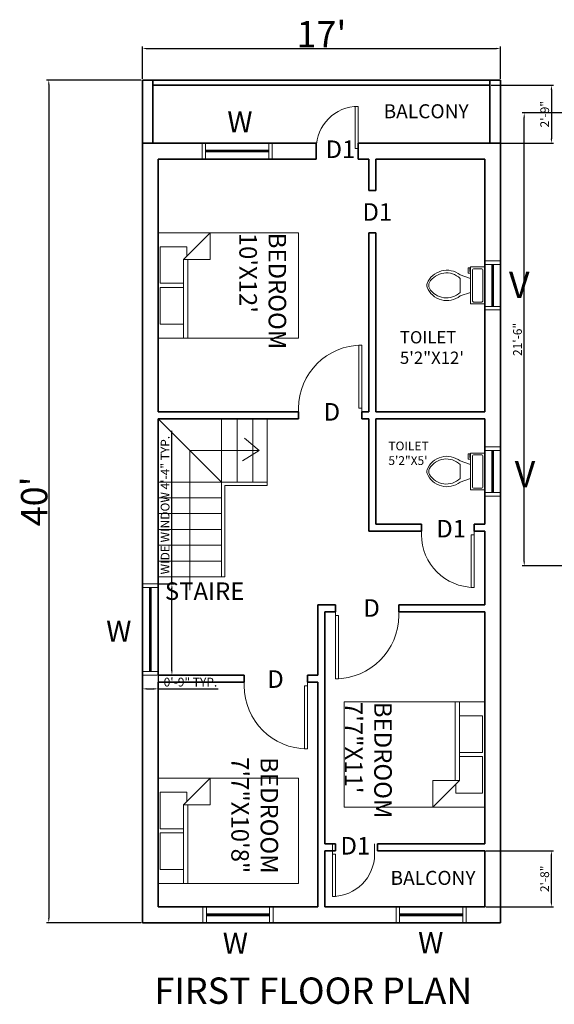
# Model space of a CAD drawing. Units: inches. Extents: x 1662 to 23131, y 1265 to 19127.
# Tile 16 of 26: x 19746 to 20050, y 8212 to 8773. Entities that reach past the tile are written whole.
import ezdxf

# ---------------------------------------------------------------- set-up
doc = ezdxf.new("R2010")
doc.units = ezdxf.units.IN
for name, color, linetype, lineweight in [('A-ANNO-DIMS', 4, 'Continuous', 18), ('A-ANNO-IDEN', 7, 'Continuous', 18), ('A-ANNO-TITL', 7, 'Continuous', 35), ('A-AREA-IDEN', 7, 'Continuous', 18), ('A-DOOR', 3, 'Continuous', 18), ('A-FLOR-FIXT', 9, 'Continuous', 18), ('A-FLOR-STRS', 7, 'Continuous', 18), ('A-FURN', 8, 'Continuous', 18), ('A-GLAZ', 4, 'Continuous', 18), ('A-WALL', 7, 'Continuous', 35)]:
    doc.layers.add(name, color=color, linetype=linetype, lineweight=lineweight)
doc.styles.get("Standard").update_dxf_attribs({"font": 'arial.ttf'})
doc.dimstyles.new('ISO-25', dxfattribs={"dimtxt": 5, "dimasz": 2.5, "dimexe": 1.25, "dimexo": 0.625, "dimtad": 1, "dimlunit": 3, "dimtxsty": 'Standard', "dimcen": 2.5, "dimadec": 0, "dimazin": 0, "dimtfac": 1, "dimtmove": 0, "dimatfit": 3, "dimfxl": 1, "dimarcsym": 0})

# ---------------------------------------------------------------- blocks, each defined once
blk = doc.blocks.new('Bed - Queen')
for p, q in [((0, -80.00003), (0, 0)), ((0, 0), (59.99999, 0)), ((59.99999, 0), (59.99999, -80.00003)), ((7.99999, -1.2), (28.79998, -1.2)), ((7.99999, -14.4), (7.99999, -1.2)), ((28.79998, -1.2), (28.79998, -14.4)), ((31.19999, -1.2), (51.99999, -1.2)), ((31.19999, -14.4), (31.19999, -1.2)), ((51.99999, -1.2), (51.99999, -16.4)), ((0, -14.4), (44.8, -14.4)), ((44.8, -16.8), (0, -16.8)), ((59.99999, -29.6), (44.8, -14.4)), ((44.8, -14.4), (44.8, -29.6)), ((51.99999, -16.4), (46.79936, -16.4)), ((44.8, -29.6), (59.99999, -29.6)), ((59.99999, -80.00003), (0, -80.00003))]:
    blk.add_line(p, q)
blk = doc.blocks.new('Toilet - top')
for p, q in [((9.5, -6), (9.5, -2)), ((-10, -8.5), (-8, -8.5)), ((-10, -9.5), (-10, -8.5)), ((-7, -9.5), (-10, -9.5)), ((-8, -8.5), (-8, -8)), ((-7, -8), (-7, -9.5)), ((-4, -8), (-6, -14)), ((4, -8), (6, -14)), ((4, -14), (-4, -14))]:
    blk.add_line(p, q)
blk.add_lwpolyline([(10.5, -8), (10.5, 0), (-10.5, 0), (-10.5, -8)], close=True)
for points in [[(-9.5, -2), (-9.5, -6)], [(8.5, -1), (-8.5, -1)], [(-8.5, -7), (8.5, -7)]]:
    blk.add_lwpolyline(points)
for centre, radius, start, end in [((-8.62, -1.88), 0.884, 81.8699, 188.1301), ((8.62, -1.88), 0.884, 351.8699, 98.1301), ((-8.62, -6.12), 0.884, 171.8699, 278.1301), ((8.62, -6.12), 0.884, 261.8699, 8.1301), ((3.52, -21.58), 12.17, 141.4691, 247.9714), ((4.2, -21.82), 11.33, 136.3677, 238.9468), ((-3.52, -21.58), 12.17, 292.0284, 38.5307), ((-4.2, -21.82), 11.33, 301.053, 43.6321), ((0, -27.88), 4, 245.7318, 294.2682), ((0, -29), 4, 254.8605, 285.1395)]:
    blk.add_arc(centre, radius, start, end)
blk = doc.blocks.new('*U87')
for p, q in [((-36, 0), (-36, 6)), ((0, 0), (0, 6))]:
    blk.add_line(p, q)
blk.add_lwpolyline([(0, 0), (0, -36), (-1.75, -36), (-1.75, 0)], close=True)
blk.add_arc((0, 0), 36, 180, 270)
blk = doc.blocks.new('*U88')
for p, q in [((0, 0), (0, 6)), ((36, 0), (36, 6))]:
    blk.add_line(p, q)
blk.add_lwpolyline([(0, 0), (0, -36), (1.75, -36), (1.75, 0)], close=True)
blk.add_arc((0, 0), 36, 270, 0)
blk = doc.blocks.new('*U89')
for p, q in [((-36, 0), (-36, -6)), ((0, 0), (0, -6))]:
    blk.add_line(p, q)
blk.add_lwpolyline([(0, 0), (0, 36), (-1.75, 36), (-1.75, 0)], close=True)
blk.add_arc((0, 0), 36, 90, 180)
blk = doc.blocks.new('*U90')
for p, q in [((0, 0), (0, 6)), ((24, 0), (24, 6))]:
    blk.add_line(p, q)
blk.add_lwpolyline([(0, 0), (0, -24), (1.75, -24), (1.75, 0)], close=True)
blk.add_arc((0, 0), 24, 270, 0)
blk = doc.blocks.new('*U91')
for p, q in [((-24, 0), (-24, -6)), ((0, 0), (0, -6))]:
    blk.add_line(p, q)
blk.add_lwpolyline([(0, 0), (0, 24), (-1.75, 24), (-1.75, 0)], close=True)
blk.add_arc((0, 0), 24, 90, 180)
blk = doc.blocks.new('*U92')
for p, q in [((-30, 0), (-30, 6)), ((0, 0), (0, 6))]:
    blk.add_line(p, q)
blk.add_lwpolyline([(0, 0), (0, -30), (-1.75, -30), (-1.75, 0)], close=True)
blk.add_arc((0, 0), 30, 180, 270)
blk = doc.blocks.new('*D96')
at = {"layer": 'A-ANNO-DIMS', "color": 0, "lineweight": -2, "transparency": 16777216}
for p, q in [((19815.56, 8739.35), (19815.56, 8757.89)), ((19818.06, 8756.64), (20017.06, 8756.64)), ((20019.56, 8739.35), (20019.56, 8757.89))]:
    blk.add_line(p, q, dxfattribs=at)
at = {"layer": 'A-ANNO-DIMS', "color": 0, "transparency": 16777216}
for points in [[(19818.06, 8757.06), (19818.06, 8756.22), (19815.56, 8756.64)], [(20017.06, 8757.06), (20017.06, 8756.22), (20019.56, 8756.64)]]:
    blk.add_solid(points, dxfattribs=at)
at = {"layer": 'Defpoints', "color": 0, "transparency": 16777216}
for p in [(20019.56, 8756.64), (19815.56, 8738.72), (20019.56, 8738.72)]:
    blk.add_point(p, dxfattribs=at)
at = {"layer": 'A-ANNO-DIMS', "color": 0, "transparency": 16777216, "insert": (19917.56, 8764.8), "char_height": 5, "attachment_point": 5}
blk.add_mtext(" {\\H3x;17'}", dxfattribs=at)
blk = doc.blocks.new('*D97')
at = {"layer": 'A-ANNO-DIMS', "color": 0, "lineweight": -2, "transparency": 16777216}
for p, q in [((19814.93, 8738.72), (19760.96, 8738.72)), ((19762.21, 8736.22), (19762.21, 8261.22)), ((19814.93, 8258.72), (19760.96, 8258.72))]:
    blk.add_line(p, q, dxfattribs=at)
at = {"layer": 'A-ANNO-DIMS', "color": 0, "transparency": 16777216}
for points in [[(19761.8, 8736.22), (19762.63, 8736.22), (19762.21, 8738.72)], [(19761.8, 8261.22), (19762.63, 8261.22), (19762.21, 8258.72)]]:
    blk.add_solid(points, dxfattribs=at)
at = {"layer": 'Defpoints', "color": 0, "transparency": 16777216}
for p in [(19815.56, 8738.72), (19762.21, 8258.72), (19815.56, 8258.72)]:
    blk.add_point(p, dxfattribs=at)
at = {"layer": 'A-ANNO-DIMS', "color": 0, "transparency": 16777216, "insert": (19753.93, 8498.72), "char_height": 5, "attachment_point": 5, "rotation": 90}
blk.add_mtext("{\\H3x;40'}", dxfattribs=at)
blk = doc.blocks.new('WIN-48-J9X2')
for p, q in [((9, 52), (0, 52)), ((9, 50), (0, 50)), ((4, 50), (4, 2)), ((4.5, 50), (4.5, 2)), ((5, 50), (5, 2)), ((9, 2), (0, 2)), ((9, 0), (0, 0))]:
    blk.add_line(p, q)
blk = doc.blocks.new('VENT-24-J9X2')
for p, q in [((9, 28), (0, 28)), ((9, 26), (0, 26)), ((4, 26), (4, 2)), ((4.5, 26), (4.5, 2)), ((5, 26), (5, 2)), ((9, 2), (0, 2)), ((9, 0), (0, 0))]:
    blk.add_line(p, q)
blk = doc.blocks.new('WIN-36-J9X2')
for p, q in [((0, 0), (0, 9)), ((2, 0), (2, 9)), ((38, 0), (38, 9)), ((40, 0), (40, 9)), ((38, 5), (2, 5)), ((38, 4.5), (2, 4.5)), ((38, 4), (2, 4))]:
    blk.add_line(p, q)
blk = doc.blocks.new('STAIR-QUARTER-TURN')
for p, q in [((36, 61.57), (0, 97.57)), ((36, 61.57), (36, 97.57)), ((45, 61.57), (45, 97.57)), ((54, 61.57), (54, 97.57)), ((62, 59.57), (62, 97.57)), ((57.46, 79.57), (49.14, 86.54)), ((18, 79.57), (18, 0)), ((18, 79.57), (57.46, 79.57)), ((57.46, 79.57), (47.96, 73.62)), ((36, 61.57), (0, 61.57)), ((36, 7.57), (36, 61.57)), ((36, 61.57), (62, 61.57)), ((38, 7.57), (38, 59.57)), ((38, 59.57), (62, 59.57)), ((36, 52.57), (0, 52.57)), ((36, 43.57), (0, 43.57)), ((36, 34.57), (0, 34.57)), ((36, 25.57), (0, 25.57)), ((36, 16.57), (0, 16.57)), ((38, 7.57), (0, 7.57))]:
    blk.add_line(p, q)
blk = doc.blocks.new('*D187')
at = {"layer": 'A-ANNO-DIMS', "color": 0, "lineweight": -2, "transparency": 16777216}
for p, q in [((19832.36, 8451.72), (19832.36, 8538.92)), ((19825.18, 8451.72), (19833.61, 8451.72)), ((19832.36, 8402.22), (19832.36, 8449.22)), ((19825.18, 8399.72), (19833.61, 8399.72))]:
    blk.add_line(p, q, dxfattribs=at)
at = {"layer": 'A-ANNO-DIMS', "color": 0, "transparency": 16777216}
for points in [[(19831.94, 8449.22), (19832.77, 8449.22), (19832.36, 8451.72)], [(19831.94, 8402.22), (19832.77, 8402.22), (19832.36, 8399.72)]]:
    blk.add_solid(points, dxfattribs=at)
at = {"layer": 'Defpoints', "color": 0, "transparency": 16777216}
for p in [(19824.56, 8451.72), (19832.36, 8451.72), (19824.56, 8399.72)]:
    blk.add_point(p, dxfattribs=at)
at = {"layer": 'A-ANNO-DIMS', "color": 0, "transparency": 16777216, "insert": (19829.14, 8496.57), "char_height": 5, "attachment_point": 5, "rotation": 90}
blk.add_mtext('WIDE WINDOW 4\'-4" TYP.', dxfattribs=at)
blk = doc.blocks.new('*D188')
at = {"layer": 'A-ANNO-DIMS', "color": 0, "lineweight": -2, "transparency": 16777216}
for p, q in [((19815.56, 8399.1), (19815.56, 8390.67)), ((19824.56, 8399.1), (19824.56, 8390.67)), ((19818.06, 8391.92), (19822.06, 8391.92)), ((19824.56, 8391.92), (19858.78, 8391.92))]:
    blk.add_line(p, q, dxfattribs=at)
at = {"layer": 'A-ANNO-DIMS', "color": 0, "transparency": 16777216}
for points in [[(19818.06, 8392.34), (19818.06, 8391.51), (19815.56, 8391.92)], [(19822.06, 8392.34), (19822.06, 8391.51), (19824.56, 8391.92)]]:
    blk.add_solid(points, dxfattribs=at)
at = {"layer": 'Defpoints', "color": 0, "transparency": 16777216}
for p in [(19815.56, 8399.72), (19824.56, 8399.72), (19824.56, 8391.92)]:
    blk.add_point(p, dxfattribs=at)
at = {"layer": 'A-ANNO-DIMS', "color": 0, "transparency": 16777216, "insert": (19842.92, 8395.1), "char_height": 5, "attachment_point": 5}
blk.add_mtext('0\'-9" TYP.', dxfattribs=at)
blk = doc.blocks.new('*D243')
at = {"layer": 'A-ANNO-DIMS', "color": 0, "lineweight": -2, "transparency": 16777216}
for p, q in [((20011.18, 8299.72), (20049.81, 8299.72)), ((20048.56, 8270.22), (20048.56, 8297.22)), ((20011.18, 8267.72), (20049.81, 8267.72))]:
    blk.add_line(p, q, dxfattribs=at)
at = {"layer": 'A-ANNO-DIMS', "color": 0, "transparency": 16777216}
for points in [[(20048.14, 8297.22), (20048.97, 8297.22), (20048.56, 8299.72)], [(20048.14, 8270.22), (20048.97, 8270.22), (20048.56, 8267.72)]]:
    blk.add_solid(points, dxfattribs=at)
at = {"layer": 'Defpoints', "color": 0, "transparency": 16777216}
for p in [(20010.56, 8299.72), (20048.56, 8299.72), (20010.56, 8267.72)]:
    blk.add_point(p, dxfattribs=at)
at = {"layer": 'A-ANNO-DIMS', "color": 0, "transparency": 16777216, "insert": (20045.38, 8283.72), "char_height": 5, "attachment_point": 5, "rotation": 90}
blk.add_mtext('2\'-8"', dxfattribs=at)
blk = doc.blocks.new('*D244')
at = {"layer": 'A-ANNO-DIMS', "color": 0, "lineweight": -2, "transparency": 16777216}
for p, q in [((20014.18, 8735.72), (20049.81, 8735.72)), ((20048.56, 8733.22), (20048.56, 8705.22)), ((20014.18, 8702.72), (20049.81, 8702.72))]:
    blk.add_line(p, q, dxfattribs=at)
at = {"layer": 'A-ANNO-DIMS', "color": 0, "transparency": 16777216}
for points in [[(20048.14, 8733.22), (20048.97, 8733.22), (20048.56, 8735.72)], [(20048.14, 8705.22), (20048.97, 8705.22), (20048.56, 8702.72)]]:
    blk.add_solid(points, dxfattribs=at)
at = {"layer": 'Defpoints', "color": 0, "transparency": 16777216}
for p in [(20013.56, 8735.72), (20013.56, 8702.72), (20048.56, 8702.72)]:
    blk.add_point(p, dxfattribs=at)
at = {"layer": 'A-ANNO-DIMS', "color": 0, "transparency": 16777216, "insert": (20045.38, 8719.22), "char_height": 5, "attachment_point": 5, "rotation": 90}
blk.add_mtext('2\'-9"', dxfattribs=at)
blk = doc.blocks.new('*D246')
at = {"layer": 'A-ANNO-DIMS', "color": 0, "lineweight": -2, "transparency": 16777216}
for p, q in [((20122.38, 8719.94), (20031.81, 8719.94)), ((20033.06, 8464.44), (20033.06, 8717.44)), ((20128.38, 8461.94), (20031.81, 8461.94))]:
    blk.add_line(p, q, dxfattribs=at)
at = {"layer": 'A-ANNO-DIMS', "color": 0, "transparency": 16777216}
for points in [[(20032.64, 8717.44), (20033.48, 8717.44), (20033.06, 8719.94)], [(20032.64, 8464.44), (20033.48, 8464.44), (20033.06, 8461.94)]]:
    blk.add_solid(points, dxfattribs=at)
at = {"layer": 'Defpoints', "color": 0, "transparency": 16777216}
for p in [(20033.06, 8719.94), (20123, 8719.94), (20129, 8461.94)]:
    blk.add_point(p, dxfattribs=at)
at = {"layer": 'A-ANNO-DIMS', "color": 0, "transparency": 16777216, "insert": (20029.88, 8590.94), "char_height": 5, "attachment_point": 5, "rotation": 90}
blk.add_mtext('21\'-6"', dxfattribs=at)

msp = doc.modelspace()

# ---------------------------------------------------------------- linework, layer by layer
at = {"layer": 'A-WALL'}
for p, q in [((19815.556, 8258.722), (19815.556, 8738.722)), ((19815.556, 8738.722), (20019.556, 8738.722)), ((19821.556, 8702.722), (19821.556, 8738.722)), ((20013.556, 8738.722), (20013.556, 8702.722)), ((20019.556, 8738.722), (20019.556, 8258.722)), ((19821.556, 8735.722), (20013.556, 8735.722)), ((19815.556, 8702.722), (19914.556, 8702.722)), ((19914.556, 8693.722), (19914.556, 8702.722)), ((19938.556, 8693.722), (19938.556, 8702.722)), ((19938.556, 8702.722), (20019.556, 8702.722)), ((19824.556, 8549.722), (19824.556, 8693.722)), ((19824.556, 8693.722), (19914.556, 8693.722)), ((19938.556, 8693.722), (19944.556, 8693.722)), ((19944.556, 8675.722), (19944.556, 8693.722)), ((19948.556, 8693.722), (20010.556, 8693.722)), ((19948.556, 8675.722), (19948.556, 8693.722)), ((20010.556, 8693.722), (20010.556, 8549.722)), ((19944.556, 8675.722), (19948.556, 8675.722)), ((19944.556, 8549.722), (19944.556, 8651.722)), ((19944.556, 8651.722), (19948.556, 8651.722)), ((19948.556, 8549.722), (19948.556, 8651.722)), ((20010.556, 8639.722), (20010.556, 8549.722)), ((19824.556, 8549.722), (19904.556, 8549.722)), ((19904.556, 8545.722), (19904.556, 8549.722)), ((19940.556, 8545.722), (19940.556, 8549.722)), ((19940.556, 8549.722), (19944.556, 8549.722)), ((19948.556, 8549.722), (20010.556, 8549.722)), ((19824.556, 8545.722), (19904.556, 8545.722)), ((19824.556, 8399.722), (19824.556, 8545.722)), ((19940.556, 8545.722), (19944.556, 8545.722)), ((19944.556, 8481.722), (19944.556, 8545.722)), ((19948.556, 8485.722), (19948.556, 8545.722)), ((19948.556, 8545.722), (20010.556, 8545.722)), ((20010.556, 8545.722), (20010.556, 8485.722)), ((20010.556, 8545.722), (20010.556, 8497.722)), ((19948.556, 8485.722), (19974.556, 8485.722)), ((19974.556, 8485.722), (19974.556, 8481.722)), ((20004.556, 8485.722), (20004.556, 8481.722)), ((20004.556, 8485.722), (20010.556, 8485.722)), ((19944.556, 8481.722), (19974.556, 8481.722)), ((20004.556, 8481.722), (20010.556, 8481.722)), ((20010.556, 8481.722), (20010.556, 8439.722)), ((19824.556, 8399.722), (19824.556, 8435.722)), ((19925.556, 8439.722), (19915.556, 8439.722)), ((19915.556, 8399.722), (19915.556, 8439.722)), ((19925.556, 8435.722), (19919.556, 8435.722)), ((19919.556, 8303.722), (19919.556, 8435.722)), ((19925.556, 8435.722), (19925.556, 8439.722)), ((20010.556, 8439.722), (19961.556, 8439.722)), ((19961.556, 8435.722), (19961.556, 8439.722)), ((20010.556, 8435.722), (19961.556, 8435.722)), ((20010.556, 8439.722), (19962.556, 8439.722)), ((20010.556, 8435.722), (20010.556, 8303.722)), ((19873.556, 8399.722), (19824.556, 8399.722)), ((19824.556, 8267.722), (19824.556, 8395.722)), ((19873.556, 8395.722), (19824.556, 8395.722)), ((19873.556, 8395.722), (19873.556, 8399.722)), ((19915.556, 8399.722), (19909.556, 8399.722)), ((19909.556, 8399.722), (19909.556, 8395.722)), ((19915.556, 8395.722), (19909.556, 8395.722)), ((19915.556, 8267.722), (19915.556, 8395.722)), ((19824.556, 8267.722), (19824.556, 8373.722)), ((19919.556, 8303.722), (19925.556, 8303.722)), ((19925.556, 8299.722), (19925.556, 8303.722)), ((19949.556, 8299.722), (19949.556, 8303.722)), ((19949.556, 8303.722), (20010.556, 8303.722)), ((19919.556, 8267.722), (19919.556, 8299.722)), ((19919.556, 8299.722), (19925.556, 8299.722)), ((19949.556, 8299.722), (20010.556, 8299.722)), ((20010.556, 8299.722), (20010.556, 8267.722)), ((19881.556, 8267.722), (19824.556, 8267.722)), ((19824.556, 8267.722), (19915.556, 8267.722)), ((19915.556, 8267.722), (19881.556, 8267.722)), ((20010.556, 8267.722), (19919.556, 8267.722)), ((19919.556, 8267.722), (20010.556, 8267.722)), ((20019.556, 8258.722), (19815.556, 8258.722))]:
    msp.add_line(p, q, dxfattribs=at)

# ---------------------------------------------------------------- block references
at = {"layer": 'A-DOOR'}
for name, p in [('*U91', (19938.556, 8699.722)), ('*U89', (19940.556, 8551.722)), ('*U92', (20004.556, 8479.722)), ('*U88', (19925.556, 8433.722)), ('*U87', (19909.556, 8393.722)), ('*U90', (19923.806, 8297.722))]:
    msp.add_blockref(name, p, dxfattribs=at)
at = {"layer": 'A-FLOR-FIXT', "rotation": 270}
for p in [(20010.556, 8621.722), (20010.556, 8515.722)]:
    msp.add_blockref('Toilet - top', p, dxfattribs=at)
at = {"layer": 'A-FLOR-STRS'}
msp.add_blockref('STAIR-QUARTER-TURN', (19824.556, 8448.15), dxfattribs=at)
at = {"layer": 'A-FURN'}
for p, rotation in [((19824.556, 8591.722), 89.99999999999999), ((20010.556, 8384.503), 270), ((19824.556, 8281.066), 89.99999999999999)]:
    msp.add_blockref('Bed - Queen', p, dxfattribs=dict(at, rotation=rotation))
at = {"layer": 'A-GLAZ'}
for name, p in [('WIN-36-J9X2', (19849.556, 8693.722)), ('VENT-24-J9X2', (20010.556, 8607.722)), ('VENT-24-J9X2', (20010.556, 8501.722)), ('WIN-48-J9X2', (19815.556, 8399.722)), ('WIN-36-J9X2', (19850.056, 8258.722)), ('WIN-36-J9X2', (19960.056, 8258.722))]:
    msp.add_blockref(name, p, dxfattribs=at)

# ---------------------------------------------------------------- texts
at = {"layer": 'A-ANNO-IDEN', "attachment_point": 1}
for s, width, heights, insert, char_height in [('W', 471.52273, [28.462], (19863.921, 8720.891), 12), ('D1', 1142.59551, [20], (19919.899, 8704.285), 10), ('D1', 1142.59551, [20], (19940.917, 8668.56), 10), ('V', 1142.59551, [20], (20024.344, 8629.571), 15), ('D', 1142.59551, [0], (19918.795, 8554.703), 10), ('V', 1142.59551, [20], (20027.618, 8521.794), 15), ('D1', 1142.59551, [20], (19982.959, 8488.152), 10), ('D', 1142.59551, [0], (19941.45, 8442.989), 10), ('W', 471.52273, [28.462], (19794.922, 8430.805), 12), ('D', 1142.59551, [0], (19886.699, 8402.479), 10), ('D1', 1142.59551, [20], (19928.412, 8307.542), 10), ('W', 471.52273, [28.462], (19861.331, 8253.024), 12), ('W', 471.52273, [28.462], (19972.636, 8253.354), 12)]:
    msp.add_mtext_dynamic_manual_height_columns(s, width=width, gutter_width=12.5, heights=heights, dxfattribs=dict(at, insert=insert, char_height=char_height))
at = {"layer": 'A-ANNO-TITL', "insert": (19822.453, 8227.504), "char_height": 15, "attachment_point": 1}
msp.add_mtext_dynamic_manual_height_columns('FIRST FLOOR PLAN', width=1142.59551, gutter_width=12.5, heights=[0], dxfattribs=at)
at = {"layer": 'A-AREA-IDEN', "attachment_point": 1}
for s, heights, insert, char_height in [('BALCONY', [0], (19952.942, 8724.911), 8), ('TOILET\\P5\'2"X12\'', [277.772], (19962.252, 8595.679), 7), ('TOILET\\P5\'2"X5\'', [277.772], (19955.677, 8532.772), 5), ('STAIRE', [0], (19828.364, 8452.561), 10), ('BALCONY', [0], (19956.883, 8288.252), 8)]:
    msp.add_mtext_dynamic_manual_height_columns(s, width=1142.59551, gutter_width=12.5, heights=heights, dxfattribs=dict(at, insert=insert, char_height=char_height))
at = {"layer": 'A-AREA-IDEN', "char_height": 10, "attachment_point": 1, "rotation": 270}
for s, insert in [("BEDROOM\\P10'X12'", (19897.451, 8651.722)), ('BEDROOM\\P7\'7"X11\'', (19957.619, 8384.503)), ('BEDROOM\\P7\'7"X10\'8"', (19892.873, 8353.04))]:
    msp.add_mtext_dynamic_manual_height_columns(s, width=1142.59551, gutter_width=12.5, heights=[277.772], dxfattribs=dict(at, insert=insert))

# ---------------------------------------------------------------- dimensions: what is measured, and where the dimension line sits
at = {"layer": 'A-ANNO-DIMS'}
for base, p1, p2, text, override, picture, middle in [((20019.556, 8756.641), (19815.556, 8738.722), (20019.556, 8738.722), ' {\\H3x;<>}', {"dimclrd": 0, "dimclre": 0, "dimclrt": 0}, '*D96', (19917.556, 8764.796)), ((19824.556, 8391.922), (19815.556, 8399.722), (19824.556, 8399.722), '<> TYP.', {"dimdec": 1, "dimlfac": 1, "dimrnd": 0, "dimzin": 1, "dimdsep": 46, "dimlunit": 4, "dimfrac": 2}, '*D188', (19842.92, 8395.1))]:
    dim = msp.add_linear_dim(base=base, p1=p1, p2=p2, text=text, dimstyle='ISO-25', override=override, dxfattribs=at)
    dim.commit()
    dim.dimension.update_dxf_attribs({"geometry": picture, "text_midpoint": middle})
for base, p1, p2, text, override, picture, middle in [((19762.214, 8258.722), (19815.556, 8738.722), (19815.556, 8258.722), '{\\H3x;<>}', {"dimclrd": 0, "dimclre": 0, "dimclrt": 0}, '*D97', (19753.931, 8498.722)), ((19832.356, 8451.722), (19824.556, 8399.722), (19824.556, 8451.722), 'WIDE WINDOW <> TYP.', {"dimdec": 1, "dimlfac": 1, "dimrnd": 0, "dimzin": 1, "dimdsep": 46, "dimlunit": 4, "dimfrac": 2}, '*D187', (19829.144, 8496.571))]:
    dim = msp.add_linear_dim(base=base, p1=p1, p2=p2, angle=90, text=text, dimstyle='ISO-25', override=override, dxfattribs=at)
    dim.commit()
    dim.dimension.update_dxf_attribs({"geometry": picture, "text_midpoint": middle})
for base, p1, p2, picture, middle in [((20048.556, 8702.722), (20013.556, 8735.722), (20013.556, 8702.722), '*D244', (20045.378, 8719.222)), ((20033.061, 8719.939), (20129.002, 8461.939), (20123.002, 8719.939), '*D246', (20029.883, 8590.939)), ((20048.556, 8299.722), (20010.556, 8267.722), (20010.556, 8299.722), '*D243', (20045.378, 8283.722))]:
    dim = msp.add_linear_dim(base=base, p1=p1, p2=p2, angle=90, dimstyle='ISO-25', override={"dimdec": 1, "dimlfac": 1, "dimrnd": 0, "dimzin": 1, "dimdsep": 46, "dimlunit": 4, "dimfrac": 2}, dxfattribs=at)
    dim.commit()
    dim.dimension.update_dxf_attribs({"geometry": picture, "text_midpoint": middle})

doc.saveas('drawing.dxf')
